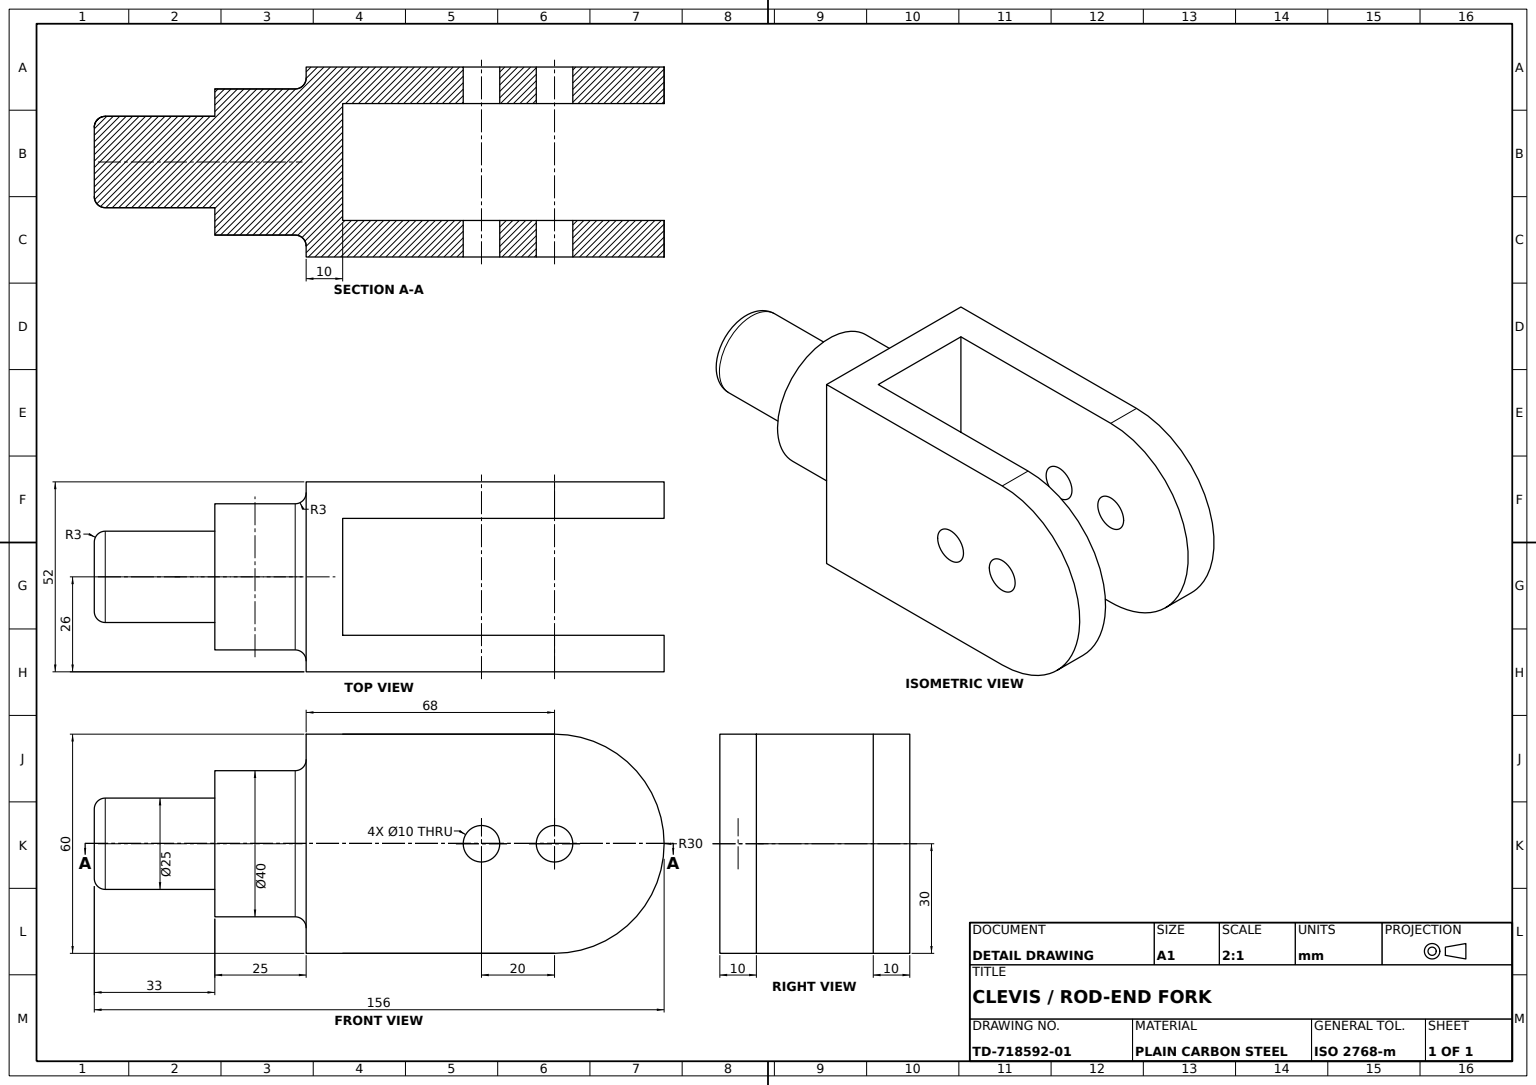
from build123d import *

# Parameters (mm, degrees)
FRONT_EAR_PROFILE_SKETCH_R = 5
FRONT_EAR_PLATE_DEPTH      = 10
BRIDGE_WALL_SKETCH_W       = 10
BRIDGE_WALL_SKETCH_H       = 42
BRIDGE_WALL_DEPTH          = 60
REAR_EAR_PROFILE_SKETCH_R  = 5
REAR_EAR_PLATE_DEPTH       = 10
COLLAR_SKETCH_26_R         = 20
SHANK_COLLAR_26_DEPTH      = 25
COLLAR_FILLET_R3_R         = 3
PIN_SHANK_SKETCH_R         = 12.5
PIN_SHANK_DEPTH            = 33
SHANK_END_FILLET_R3_R      = 3


with BuildPart() as part:
    # Front Ear Profile Sketch → Front Ear Plate (new body)
    with BuildSketch(Plane.XY):
        with BuildLine():
            Line((0, 0), (68, 0))
            ThreePointArc((68, 0), (98, 30), (68, 60))
            Line((68, 60), (0, 60))
            Line((0, 60), (0, 0))
        make_face()
        with Locations((68, 30)):
            Circle(FRONT_EAR_PROFILE_SKETCH_R, mode=Mode.SUBTRACT)
        with Locations((48, 30)):
            Circle(FRONT_EAR_PROFILE_SKETCH_R, mode=Mode.SUBTRACT)
    extrude(amount=FRONT_EAR_PLATE_DEPTH)

    # Bridge Wall Sketch → Bridge Wall (add)
    with BuildSketch(Plane(origin=(0, 60, 0), x_dir=(1, 0, 0), z_dir=(0, 1, 0))):
        with Locations((5, 21)):
            Rectangle(BRIDGE_WALL_SKETCH_W, BRIDGE_WALL_SKETCH_H)
    extrude(amount=-BRIDGE_WALL_DEPTH)

    # Rear Ear Profile Sketch → Rear Ear Plate (add)
    with BuildSketch(Plane(origin=(0, 0, -42), x_dir=(-1, 0, 0), z_dir=(0, 0, -1))):
        with BuildLine():
            Line((-10, 60), (-68, 60))
            ThreePointArc((-68, 60), (-98, 30), (-68, 0))
            Line((-68, 0), (-10, 0))
            Line((-10, 0), (-10, 60))
        make_face()
        with Locations(Location((-68, 30, 0), (0, 0, 180))):
            Circle(REAR_EAR_PROFILE_SKETCH_R, mode=Mode.SUBTRACT)
        with Locations(Location((-48, 30, 0), (0, 0, 180))):
            Circle(REAR_EAR_PROFILE_SKETCH_R, mode=Mode.SUBTRACT)
    extrude(amount=-REAR_EAR_PLATE_DEPTH)

    # Collar Sketch Ø26 → Shank Collar Ø26 (add)
    with BuildSketch(Plane.ZY):
        with Locations((-16, 30)):
            Circle(COLLAR_SKETCH_26_R)
    extrude(amount=SHANK_COLLAR_26_DEPTH)

    # Collar Fillet R3
    collar_fillet_r3_edges = [part.edges().sort_by_distance(p)[0] for p in [
        (0, 30, -36),
    ]]
    fillet(collar_fillet_r3_edges, radius=COLLAR_FILLET_R3_R)

    # Pin Shank Sketch → Pin Shank (add)
    with BuildSketch(Plane.ZY.offset(25)):
        with Locations((-16, 30)):
            Circle(PIN_SHANK_SKETCH_R)
    extrude(amount=PIN_SHANK_DEPTH)

    # Shank End Fillet R3
    shank_end_fillet_r3_edges = [part.edges().sort_by_distance(p)[0] for p in [
        (-58, 30, -28.5),
    ]]
    fillet(shank_end_fillet_r3_edges, radius=SHANK_END_FILLET_R3_R)


solid = part.part
